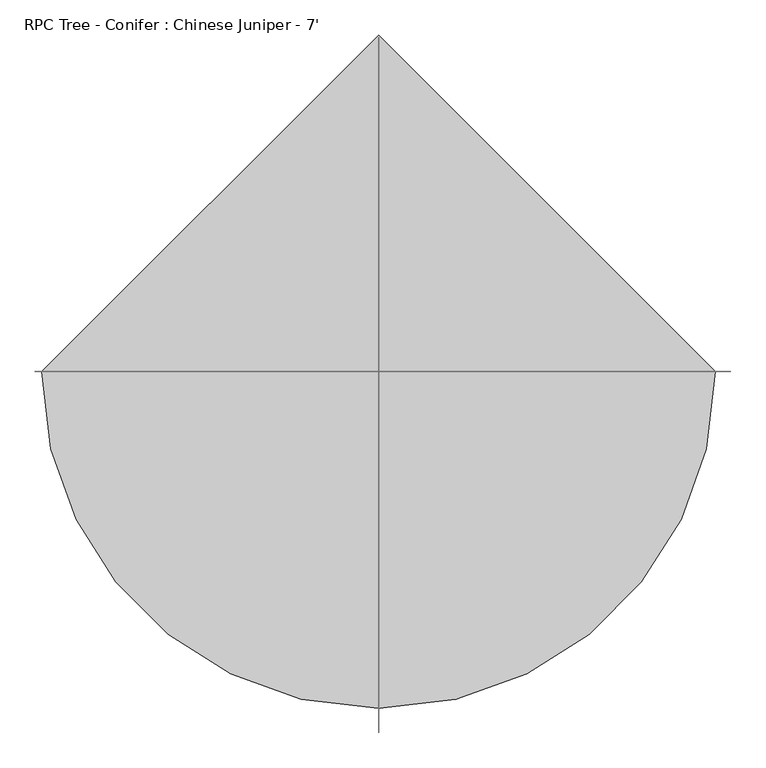
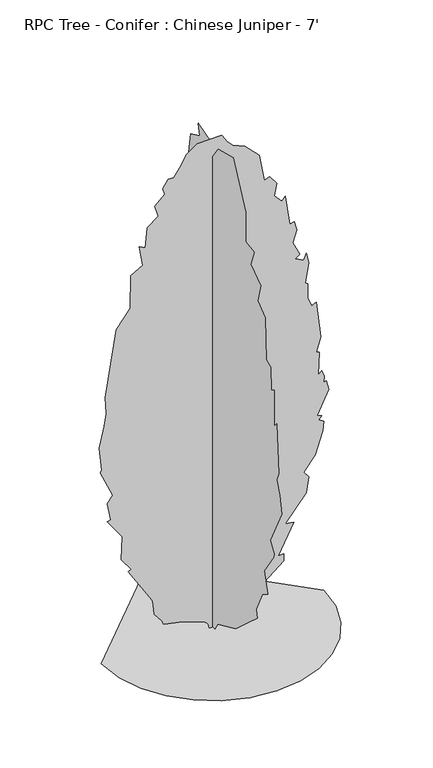
"""IFC4 building model written with IfcOpenShell, lengths in millimetres: geographic element geometry, RPC Tree - Conifer : Chinese Juniper - 7'."""

from ifc_helpers import new_model, si_unit, origin, place, context, project, spatial, triangles, source, transform, mapped, element, save


def rpc_tree_conifer_chinese_juniper_7_5155a079(model_context):
    return source(origin(), model_context, "Body", "Tessellation", [
        triangles([(-20.8237834, 9e-07, 1.9e-06), (-25.8087308, -4e-07, 25.6281368), (-39.2590862, -9e-07, 43.4163588), (-176.6107678, 2.1e-06, 93.9654218), (-288.192965, 5.6e-06, 117.6426557), (-298.8878427, 4.5e-06, 144.3795048), (-341.9790533, 3.1e-06, 199.5412178), (-352.3622495, -1.5e-06, 283.4115708), (-368.4056743, -2.7e-06, 315.4958588), (-496.7414091, -9.2e-06, 518.6950473), (-480.1370084, -1.05e-05, 528.6736533), (-536.920679, -1.28e-05, 608.2775153), (-531.1657614, -2.14e-05, 749.4692968), (-619.7322304, -2.49e-05, 871.625576), (-598.3417119, -2.61e-05, 876.9704533), (-618.9013218, -3.17e-05, 985.0297005), (-587.6446541, -3.55e-05, 1026.6967066), (-662.5096338, -4.21e-05, 1192.4684921), (-651.8161732, -4.32e-05, 1203.1619528), (-667.8581446, -5.11e-05, 1347.5396954), (-638.8367329, -5.99e-05, 1473.5058437), (-625.0771803, -6.48e-05, 1545.395351), (-630.425691, -7.06e-05, 1646.9956902), (-566.2578054, -9.73e-05, 2048.0485359), (-486.0479485, -0.0001072, 2154.9973858), (-481.7118032, -0.0001193, 2354.6093296), (-411.1830414, -0.0001248, 2395.6303722), (-432.5735235, -0.0001312, 2518.6174873), (-396.0663405, -0.0001316, 2497.6734169), (-384.4476457, -0.0001394, 2620.2179718), (-320.2772166, -0.000145, 2668.3438133), (-341.6670084, -0.0001482, 2737.8602097), (-282.845508, -0.000154, 2791.3345619), (-293.5404038, -0.0001558, 2828.7671608), (-261.4560977, -0.00016, 2876.8930023), (-229.3718097, -0.0001614, 2876.8930023), (-192.5598307, -0.0001659, 2924.6886314), (-155.6542527, -0.0001716, 2994.0672455), (-89.4394898, -0.0001772, 3038.905497), (52.9363128, -0.0001836, 3041.1446045), (86.1240581, -0.0001819, 2989.1867294), (118.2083552, -0.0001814, 2957.102932), (189.5408471, -0.0001827, 2926.891404), (273.2823744, -0.0001812, 2839.4606941), (305.3666805, -0.0001727, 2673.6923241), (337.4509867, -0.0001747, 2684.3858574), (376.5823554, -0.0001731, 2628.4041), (364.1871091, -0.0001683, 2556.0500862), (406.9681097, -0.0001673, 2507.9242447), (428.3549583, -0.0001695, 2529.3147995), (455.0939876, -0.0001598, 2347.5008972), (481.8293833, -0.0001613, 2352.849408), (496.3691208, -0.0001588, 2299.8757519), (472.4712699, -0.0001534, 2227.184404), (513.9133261, -0.0001499, 2138.9553417), (485.8934157, -0.0001477, 2122.1550591), (535.3038082, -0.0001483, 2096.1743774), (551.3457796, -0.0001513, 2133.606831), (567.387751, -0.0001481, 2069.4389454), (546.0009024, -0.0001402, 1951.7967075), (561.4405123, -0.0001401, 1939.0929771), (559.2960211, -0.0001348, 1852.232), (583.4297224, -0.0001326, 1796.7218708), (610.1687153, -0.0001344, 1807.4154041), (636.9040747, -0.0001222, 1582.8278046), (610.1687153, -0.0001159, 1497.2695095), (626.8202425, -0.0001163, 1491.6125874), (620.8621759, -0.0001078, 1352.8882061), (642.2526581, -0.0001097, 1368.9301048), (658.2946295, -0.0001081, 1331.4976513), (652.9460461, -0.0001057, 1294.0688313), (668.9880175, -0.0001067, 1299.4137085), (685.0299889, -0.0001039, 1240.5943336), (615.5135925, -9.26e-05, 1101.5616137), (642.2526581, -9.31e-05, 1090.868153), (626.2106867, -9.11e-05, 1069.4776709), (652.9460461, -9.13e-05, 1053.4356995), (647.3217527, -8.76e-05, 995.8029528), (604.8202045, -7.77e-05, 860.9284819), (535.3038082, -6.96e-05, 775.3701141), (567.387751, -6.88e-05, 737.9376606), (549.8508127, -6.24e-05, 644.5234497), (428.3549583, -4.8e-05, 491.9596516), (476.484506, -4.98e-05, 486.6111408), (385.5775912, -3.53e-05, 310.1484017), (417.661534, -3.67e-05, 310.1484017), (417.661534, -3.42e-05, 267.369236), (182.3762044, -1.24e-05, 74.8634718), (182.3762044, -1.4e-05, 101.600321), (21.9553232, -1e-06, 0.0), (0.1966726, 19.6988158, 0.0001857), (0.1966748, 49.2587393, 20.4233355), (0.1966784, 110.6042953, 42.7795427), (0.1966813, 254.9838002, 96.2532454), (0.1966876, 329.847272, 165.7692784), (0.1966865, 297.762984, 171.1167173), (0.1966987, 412.2070341, 336.0808305), (0.1967007, 377.9749666, 417.0947445), (0.1967053, 474.2267587, 556.1275372), (0.1967076, 463.5333344, 620.2953501), (0.1967144, 533.0460972, 705.8537178), (0.1967199, 556.4178174, 808.187079), (0.1967182, 543.743155, 914.4029068), (0.1967276, 629.3015591, 1042.738678), (0.1967334, 634.6464363, 1171.07801), (0.1967367, 603.7599495, 1276.1036488), (0.1967403, 650.6884077, 1443.7950119), (0.196741, 607.9110406, 1502.6143867), (0.1967462, 554.4366157, 1673.7311222), (0.1967472, 591.8690692, 1791.3733601), (0.1967528, 549.0880686, 1962.4900955), (0.1967549, 495.6172771, 2064.0904346), (0.1967574, 468.8782479, 2277.9881344), (0.1967553, 436.7943051, 2261.9462357), (0.1967637, 436.7943051, 2454.4498924), (0.1967616, 372.6264559, 2470.4916458), (0.1967594, 338.6788914, 2584.7195572), (0.1967626, 319.1523943, 2679.0408348), (0.1967626, 254.9838002, 2743.2087204), (0.1967696, 222.899494, 2935.7158653), (0.1967618, 131.9936965, 2978.4934868), (0.1967654, 145.7997306, 3047.3276573), (0.1967579, 16.2125085, 3006.0162254), (0.1967593, 9.0039295, 2914.3256012), (0.1967548, -55.1646243, 3005.2322617), (0.1967499, -210.2386571, 3048.0098831), (0.1967385, -338.5761724, 2785.9860512), (0.1967306, -338.5761724, 2604.1759277), (0.1967262, -423.1508429, 2589.1210327), (0.1967236, -386.7017232, 2491.8822006), (0.1967217, -489.7752645, 2421.5203617), (0.1967181, -461.5666666, 2310.0720772), (0.1967123, -536.4279402, 2251.2490688), (0.1967063, -547.124998, 1994.5740383), (0.1967036, -590.7841063, 1975.9485764), (0.1966972, -595.2509122, 1834.1543243), (0.1966967, -627.3348186, 1855.5412457), (0.1966926, -627.3348186, 1630.9537914), (0.1966871, -654.0702507, 1663.0377342), (0.1966789, -675.4607328, 1363.5852276), (0.1966776, -652.2414379, 1312.6508366), (0.1966728, -686.157827, 1235.2458229), (0.1966731, -702.1997257, 1128.2970457), (0.196668, -589.9023651, 898.3609354), (0.1966635, -627.3348186, 834.1931225), (0.1966684, -624.1706949, 811.539854), (0.1966665, -525.7345159, 668.4248978), (0.1966595, -563.1669694, 545.4340765), (0.1966604, -504.3439974, 508.001623), (0.1966631, -445.5246952, 379.6658881), (0.1966605, -456.2181195, 331.5381935), (0.196661, -349.2707231, 235.2853114), (0.1966615, -236.9755062, 133.6849814), (0.1966659, -49.8164542, 48.1266227), (0.1966707, -23.0802909, 0.0001832), (-654.3235056, 0.0, 0.0002131), (-637.0188206, -149.9726046, 0.0002035), (-587.7390161, -287.6987364, 0.0001931), (-510.4284007, -409.231598, 0.0001825), (-409.0349167, -510.625082, 0.000172), (-287.5020733, -587.9356974, 0.0001621), (-149.7759323, -637.2154655, 0.0001531), (0.1967005, -654.5201506, 0.0001455), (150.1692768, -637.2154655, 0.00014), (287.8953996, -587.9356974, 0.0001369), (409.4282793, -510.625082, 0.0001362), (510.8217633, -409.231598, 0.0001378), (588.1323787, -287.6983731, 0.0001417), (637.4121105, -149.9726046, 0.0001477), (654.7167955, 5.72e-05, 0.0001559), (0.1965856, 654.5201506, 0.0002236)], [[57, 58, 59], [27, 28, 29], [87, 88, 89], [49, 50, 51], [13, 14, 15], [83, 84, 85], [74, 75, 76], [63, 64, 65], [68, 69, 70], [71, 72, 73], [9, 10, 11], [85, 86, 87], [85, 87, 89], [51, 52, 53], [54, 55, 56], [90, 1, 2], [66, 67, 68], [45, 46, 47], [17, 18, 19], [68, 70, 71], [45, 47, 48], [31, 32, 33], [76, 77, 78], [89, 90, 2], [89, 2, 3], [57, 59, 60], [51, 53, 54], [25, 26, 27], [39, 40, 41], [56, 57, 60], [71, 73, 74], [34, 35, 36], [33, 34, 36], [4, 5, 6], [60, 61, 62], [80, 81, 82], [38, 39, 41], [37, 38, 41], [37, 41, 42], [29, 30, 31], [15, 16, 17], [36, 37, 42], [33, 36, 42], [31, 33, 42], [31, 42, 43], [31, 43, 44], [31, 44, 45], [29, 31, 45], [29, 45, 48], [27, 29, 48], [25, 27, 48], [25, 48, 49], [25, 49, 51], [25, 51, 54], [25, 54, 56], [25, 56, 60], [25, 60, 62], [24, 25, 62], [23, 24, 62], [22, 23, 62], [22, 62, 63], [22, 63, 65], [22, 65, 66], [22, 66, 68], [21, 22, 68], [20, 21, 68], [19, 20, 68], [17, 19, 68], [17, 68, 71], [17, 71, 74], [15, 17, 74], [13, 15, 74], [13, 74, 76], [13, 76, 78], [13, 78, 79], [13, 79, 80], [12, 13, 80], [11, 12, 80], [9, 11, 80], [9, 80, 82], [9, 82, 83], [9, 83, 85], [9, 85, 89], [9, 89, 3], [9, 3, 4], [8, 9, 4], [8, 4, 6], [7, 8, 6], [138, 139, 140], [94, 95, 96], [136, 137, 138], [121, 122, 123], [112, 113, 114], [128, 129, 130], [121, 123, 124], [125, 126, 127], [124, 125, 127], [114, 115, 116], [147, 148, 149], [130, 131, 132], [124, 127, 128], [134, 135, 136], [154, 155, 91], [154, 91, 92], [150, 151, 152], [96, 97, 98], [119, 120, 121], [119, 121, 124], [119, 124, 128], [118, 119, 128], [117, 118, 128], [116, 117, 128], [116, 128, 130], [114, 116, 130], [114, 130, 132], [112, 114, 132], [112, 132, 133], [112, 133, 134], [112, 134, 136], [111, 112, 136], [110, 111, 136], [109, 110, 136], [109, 136, 138], [109, 138, 140], [109, 140, 141], [108, 109, 141], [107, 108, 141], [106, 107, 141], [105, 106, 141], [104, 105, 141], [103, 104, 141], [103, 141, 142], [103, 142, 143], [103, 143, 144], [102, 103, 144], [101, 102, 144], [100, 101, 144], [100, 144, 145], [100, 145, 146], [100, 146, 147], [100, 147, 149], [100, 149, 150], [100, 150, 152], [100, 152, 153], [100, 153, 154], [99, 100, 154], [98, 99, 154], [96, 98, 154], [96, 154, 92], [96, 92, 93], [96, 93, 94], [170, 171, 156], [169, 170, 156], [169, 156, 157], [168, 169, 157], [168, 157, 158], [168, 158, 159], [167, 168, 159], [166, 167, 159], [166, 159, 160], [166, 160, 161], [166, 161, 162], [166, 162, 163], [166, 163, 164], [166, 164, 165]], closed=False),
    ])


if __name__ == "__main__":
    model = new_model("IFC4")
    model_context = context("Model", 3, world=origin())
    ifc_project = project(units=[si_unit("LENGTHUNIT", "METRE", prefix="MILLI")], contexts=[model_context])
    site = spatial("IfcSite", under=ifc_project)
    building = spatial("IfcBuilding", under=site)
    placement = place(None, origin())
    rpc_tree_conifer_chinese_juniper_7_shape = rpc_tree_conifer_chinese_juniper_7_5155a079(model_context)
    element("IfcGeographicElement", 1, ObjectType="RPC Tree - Conifer : Chinese Juniper - 7'", at=placement, inside=building, context=model_context, shape_type="MappedRepresentation", body=[
        mapped(rpc_tree_conifer_chinese_juniper_7_shape, transform((0.0, 0.0, 0.0), x_axis=(1.0, 0.0, 0.0), y_axis=(0.0, 1.0, 0.0), z_axis=(0.0, 0.0, 1.0))),
    ])
    save(model, "model.ifc")

# Revit data of these elements
# Type "RPC Tree - Conifer : Chinese Juniper - 7'"
#   built-in parameter 1005198 = "{2, 15},{39, RPC-16-FUM3-UUQ0-UBF0-N000-ST1L-LVER-AU},{1, 0},{1, 0},{2, 13},{1, 8},{5, Color},{1, 0},{1, 0},{3, 0.8},{3, 0.8},{3, 0.8},{1, 8},{7, BBoxMin},{1, 0},{1, 0},{1, 0},{1, 0},{1, 0},{1, 8},{7, BBoxMax},{1, 0},{1, 0},{1, 0},{1, 0},{1, 0},{2, 11},{9, RPCTypeId},{1, 0},{1, 0},{39, RPC-16-FUM3-UUQ0-UBF0-N000-ST1L-LVER-AU},{1, 6},{14, RPCPlantHeight},{1, 0},{1, 0},{1, 7},{2, 11},{7, keyword},{1, 0},{1, 0},{34, :RPCs:Trees [General]:Geometry:RPC},{2, 11},{8, category},{1, 0},{1, 0},{15, Trees [General]},{2, 11},{12, LocalizedUID},{1, 0},{1, 0},{15, Chinese Juniper},{2, 14},{6, Height},{1, 0},{1, 0},{1, 7},{1, 2},{16, Cast Reflections},{1, 0},{1, 0},{1, 0},{1, 2},{12, Cast Shadows},{1, 0},{1, 0},{1, 1},{1, 2},{9, Lock View},{1, 0},{1, 0},{1, 0},{1, 4},{5, ViewC},{1, 0},{1, 0},{1, 0},{21, assetlibrary_base.fbx},{1, 5},"
#   built-in parameter 1005195 = "RPC-16-FUM3-UUQ0-UBF0-N000-ST1L-LVER-AU"
#   Type Comments = "Chinese Juniper"
#   Assembly Code = "G2050500"
#   Height = 10' - 0"
#   Description = (empty or 0)
#   Default Elevation = 0
